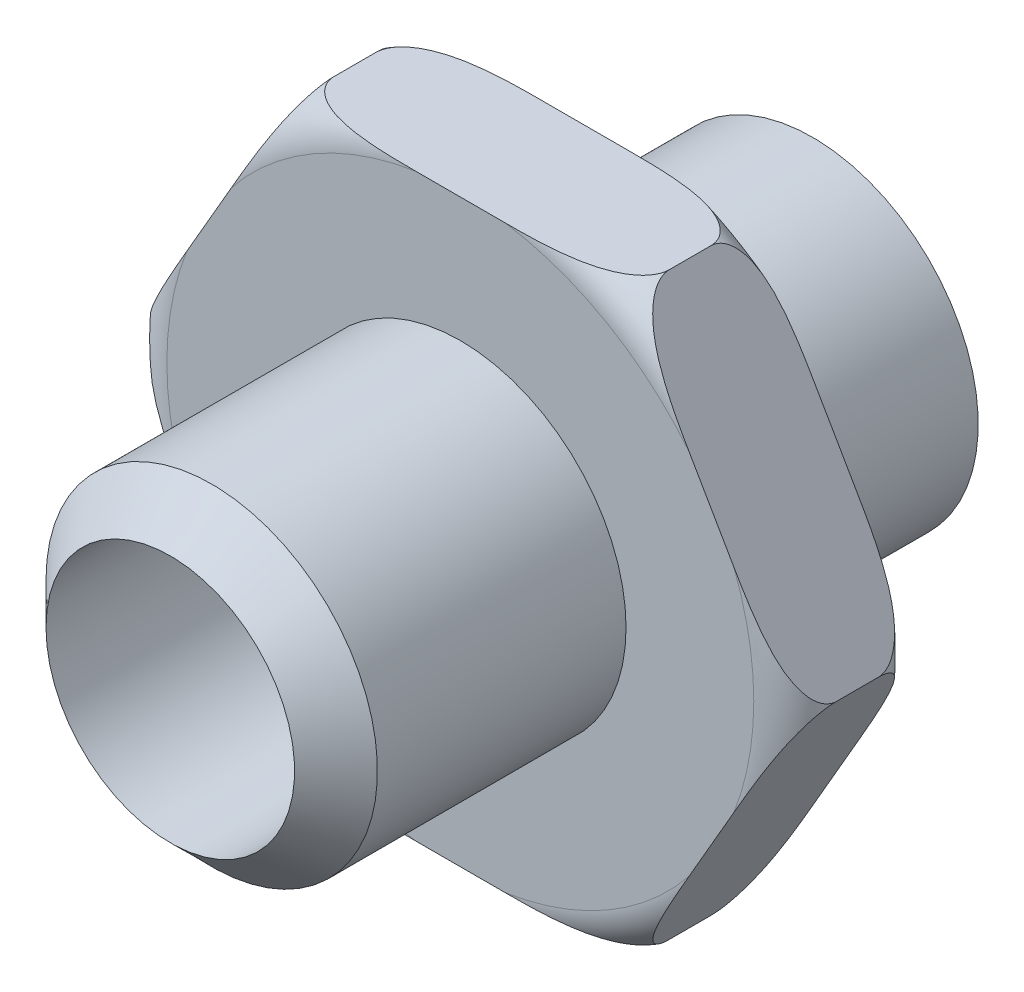
from build123d import *

# Parameters (mm, degrees)
HEX_BODY_28_DEPTH        = 6
SPIGOT_CHAMFER_3X45_SIZE = 3
THROUGH_BORE_10_REACH    = 40.488
BORE_SKETCH_10_R         = 6


with BuildPart() as part:
    # Hex Profile Sketch → Hex Body 28 (new body)
    with BuildSketch(Plane.XY):
        Polygon((8.082903769, 14), (-8.082903769, 14), (-16.165807537, 0), (-8.082903769, -14), (8.082903769, -14), (16.165807537, 0), align=None)
    extrude(amount=-HEX_BODY_28_DEPTH)

    # Spigot Profile Sketch → Threaded Spigots (revolve)
    with BuildSketch(Plane(origin=(0, 0, 0), x_dir=(1, 0, 0), z_dir=(0, 1, 0))):
        Polygon((0, 17), (-8, 17), (-8, -7), (-8, -15), (0, -15), align=None)
    revolve(axis=Axis((0, 0, -19.030185158), (0, 0, 1)))

    # Spigot Chamfer 3x45
    spigot_chamfer_3x45_edges = [part.edges().sort_by_distance(p)[0] for p in [
        (8, 0, 15),
    ]]
    chamfer(spigot_chamfer_3x45_edges, length=SPIGOT_CHAMFER_3X45_SIZE)

    # Through Bore Ø10: up to this cone (the profile starts inside it)
    through_bore_10_end = Plane(origin=(0, 0, -17), z_dir=(0, 0, -1)).offset(-36.999999) * Cone(1e-06, 114.988, 114.987999, align=(Align.CENTER, Align.CENTER, Align.MIN), mode=Mode.PRIVATE)
    # Bore Sketch Ø10 → Through Bore Ø10 (cut, up to the surface)
    with BuildSketch(Plane(origin=(0, 0, -17), x_dir=(-1, 0, 0), z_dir=(0, 0, -1)), mode=Mode.PRIVATE) as through_bore_10_sk1:
        Circle(BORE_SKETCH_10_R)
    through_bore_10_tool1 = extrude(through_bore_10_sk1.sketch, amount=-THROUGH_BORE_10_REACH, mode=Mode.PRIVATE) & through_bore_10_end
    add(through_bore_10_tool1.solids().sort_by_distance((0, 0, -17))[0], mode=Mode.SUBTRACT)

    # Thread Groove Profile Sketch → Thread Grooves (revolve, cut)
    with BuildSketch(Plane(origin=(0, 0, 0), x_dir=(1, 0, 0), z_dir=(0, 1, 0))):
        with BuildLine():
            Line((-14.165807537, 6), (-16.165807537, 6))
            Line((-16.165807537, 6), (-16.165807537, 4))
            ThreePointArc((-16.165807537, 4), (-15.5800211, 5.414213562), (-14.165807537, 6))
        make_face()
        with BuildLine():
            Line((-16.165807537, 0), (-16.165807537, 2))
            ThreePointArc((-16.165807537, 2), (-15.5800211, 0.585786438), (-14.165807537, 0))
            Line((-14.165807537, 0), (-16.165807537, 0))
        make_face()
    revolve(axis=Axis((0, 0, 0), (0, 0, -1)), mode=Mode.SUBTRACT)


solid = part.part
